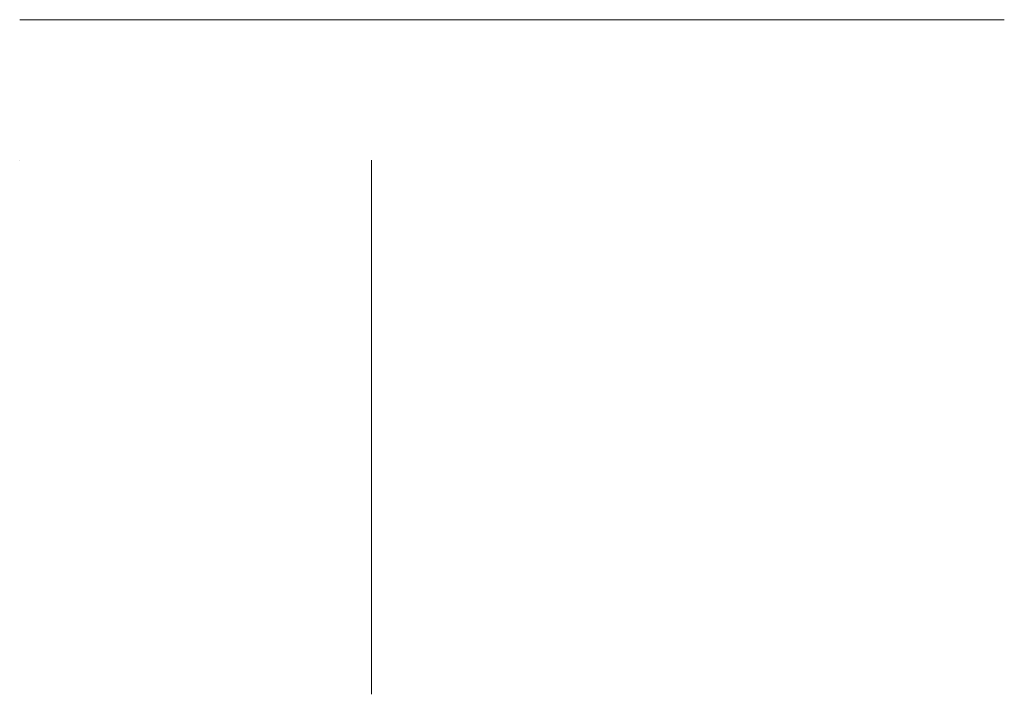
# Model space of a CAD drawing. Units: millimetres. Extents: x 439 to 579, y -96 to 0.
import ezdxf

# ---------------------------------------------------------------- set-up
doc = ezdxf.new("R2010")
doc.units = ezdxf.units.MM
doc.layers.add('M-CONS', color=8, linetype='Continuous', lineweight=18)

msp = doc.modelspace()

# ---------------------------------------------------------------- linework, layer by layer
at = {"layer": 'M-CONS', "extrusion": (0, -1, 0)}
for p, q in [((470.5, 0, 232.96), (438.5, 0, 232.96)), ((438.5, 0, 232.96), (438.5, 0, 288.96)), ((438.5, 0, 232.96), (454.5, 0, 232.96)), ((470.5, 0, 316.96), (470.5, 0, 280.96)), ((470.5, 0, 280.96), (470.5, 0, 232.96)), ((492.5, 0, 232.96), (470.5, 0, 232.96)), ((508.5, 0, 280.96), (492.5, 0, 280.96)), ((492.5, 0, 280.96), (492.5, 0, 232.96)), ((508.5, 0, 280.96), (524.5, 0, 280.96)), ((524.5, 0, 280.96), (524.5, 0, 232.96)), ((524.5, 0, 232.96), (546.5, 0, 232.96)), ((546.5, 0, 316.96), (546.5, 0, 280.96)), ((546.5, 0, 280.96), (546.5, 0, 232.96)), ((546.5, 0, 232.96), (578.5, 0, 232.96)), ((578.5, 0, 232.96), (562.5, 0, 232.96)), ((578.5, 0, 232.96), (578.5, 0, 288.96)), ((438.5, -20, 232.96), (438.5, -20, 280.96))]:
    msp.add_line(p, q, dxfattribs=at)
at = {"layer": 'M-CONS', "extrusion": (-1, 0, 0), "elevation": -488.5}
msp.add_lwpolyline([(80, 232.96, 1), (80, 264.96), (34, 248.96), (34.82, 277), (20, 280.96), (20, 248.96), (20, 232.96)], format="xyb", close=True, dxfattribs=at)
at = {"layer": 'M-CONS'}
msp.add_polyline3d([(492.5, 0, 232.96), (524.5, 0, 232.96), (524.5, 0, 280.96), (492.5, 0, 280.96)], close=True, dxfattribs=at)
at = {"layer": 'M-CONS', "extrusion": (0, -1, 0)}
for centre, radius in [((454.5, 246.96), 8), ((454.5, 274.96), 8), ((508.5, 316.96), 20), ((562.5, 246.96), 8), ((562.5, 274.96), 8)]:
    msp.add_circle(centre, radius, dxfattribs=at)
at = {"layer": 'M-CONS', "extrusion": (-1, 0, 0)}
msp.add_circle((80, 248.96, -488.5), 8, dxfattribs=at)
at = {"layer": 'M-CONS', "extrusion": (0, -1, 0)}
for centre, radius, start, end in [((442.5, 316.67), 28, 261.7837, 0.5881), ((508.5, 316.96), 38, 0, 180), ((574.5, 316.67), 28, 179.4119, 278.2163)]:
    msp.add_arc(centre, radius, start, end, dxfattribs=at)

doc.saveas('drawing.dxf')
